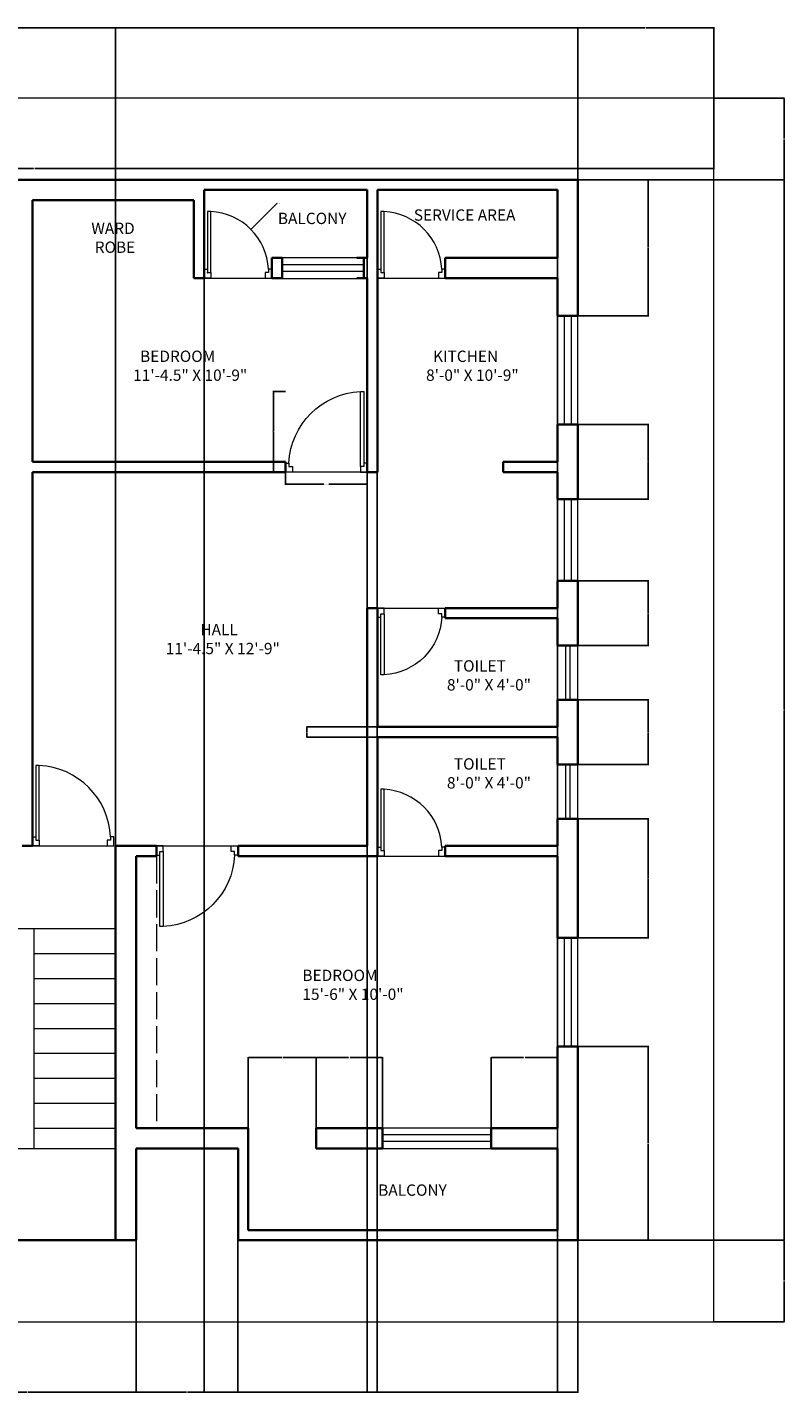
# Model space of a CAD drawing. Units: inches. Extents: x 3263 to 3926, y 954 to 1556.
# Tile 3 of 3: x 3592 to 3926, y 954 to 1556. Entities that reach past the tile are written whole.
import ezdxf

# ---------------------------------------------------------------- set-up
doc = ezdxf.new("R2010")
doc.units = ezdxf.units.IN
doc.linetypes.add('ACAD_ISO02W100', pattern=[15, 12, -3])
for name, color, linetype, lineweight in [('A-ANNO-DIMS', 2, 'Continuous', 18), ('A-ANNO-TEXT', 7, 'Continuous', 18), ('A-AREA-IDEN', 7, 'Continuous', 18), ('A-FLOR-OVHD', 8, 'ACAD_ISO02W100', 13), ('C-PROP', 8, 'Continuous', 18), ('door', 30, 'Continuous', 18), ('staircase', 31, 'Continuous', 18), ('ventilator', 210, 'Continuous', 18), ('wall', 7, 'Continuous', 35), ('window', 92, 'Continuous', 18)]:
    doc.layers.add(name, color=color, linetype=linetype, lineweight=lineweight)
doc.styles.get("Standard").update_dxf_attribs({"font": 'arial.ttf'})
doc.dimstyles.get("Standard").update_dxf_attribs({"dimtxt": 0.18, "dimasz": 0.18, "dimexe": 0.18, "dimexo": 0.0625, "dimgap": 0.09, "dimtad": 0, "dimtih": 1, "dimtoh": 1, "dimdec": 4, "dimzin": 0, "dimdsep": 46, "dimtxsty": 'Standard', "dimcen": 0.09, "dimadec": 0, "dimazin": 0, "dimtfac": 1, "dimtdec": 4, "dimtofl": 0, "dimtmove": 0, "dimatfit": 3, "dimfxl": 1, "dimtolj": 1, "dimtzin": 0, "dimarcsym": 0})

# ---------------------------------------------------------------- blocks, each defined once
blk = doc.blocks.new('d1')
at = {"layer": 'door'}
blk.add_line((4131.56, 1272.79), (4167.56, 1272.79), dxfattribs=at)
blk.add_lwpolyline([(4133.06, 1275.29), (4134.56, 1275.29), (4134.56, 1308.29), (4133.06, 1308.29)], close=True, dxfattribs=at)
for points in [[(4134.56, 1272.79), (4131.56, 1272.79), (4131.56, 1276.79), (4133.06, 1276.79), (4133.06, 1275.29), (4134.56, 1275.29), (4134.56, 1272.79)], [(4164.56, 1272.79), (4167.56, 1272.79), (4167.56, 1276.79), (4166.06, 1276.79), (4166.06, 1275.29), (4164.56, 1275.29), (4164.56, 1272.79)]]:
    blk.add_lwpolyline(points, dxfattribs=at)
blk.add_arc((4133.06, 1275.29), 33.03, 2.60256, 87.39744, dxfattribs=at)
blk = doc.blocks.new('w1')
at = {"layer": 'window'}
for p, q in [((3981.35, 1421.04), (3981.35, 1373.04)), ((3984.35, 1421.04), (3984.35, 1373.04))]:
    blk.add_line(p, q, dxfattribs=at)
blk.add_lwpolyline([(3978.35, 1373.04), (3987.35, 1373.04), (3987.35, 1421.04), (3978.35, 1421.04)], close=True, dxfattribs=at)
blk = doc.blocks.new('w2')
at = {"layer": 'window'}
for p, q in [((4050.84, 1450.41), (4050.84, 1414.41)), ((4053.84, 1450.41), (4053.84, 1414.41))]:
    blk.add_line(p, q, dxfattribs=at)
blk.add_lwpolyline([(4047.84, 1414.41), (4056.84, 1414.41), (4056.84, 1450.41), (4047.84, 1450.41)], close=True, dxfattribs=at)
blk = doc.blocks.new('d2')
at = {"layer": 'door'}
blk.add_line((4131.56, 1215.38), (4161.56, 1215.38), dxfattribs=at)
blk.add_lwpolyline([(4133.06, 1217.88), (4134.56, 1217.88), (4134.56, 1244.88), (4133.06, 1244.88)], close=True, dxfattribs=at)
for points in [[(4134.56, 1215.38), (4131.56, 1215.38), (4131.56, 1219.38), (4133.06, 1219.38), (4133.06, 1217.88), (4134.56, 1217.88), (4134.56, 1215.38)], [(4158.56, 1215.38), (4161.56, 1215.38), (4161.56, 1219.38), (4160.06, 1219.38), (4160.06, 1217.88), (4158.56, 1217.88), (4158.56, 1215.38)]]:
    blk.add_lwpolyline(points, dxfattribs=at)
blk.add_arc((4133.06, 1217.88), 27.04, 3.17983, 86.82017, dxfattribs=at)
blk = doc.blocks.new('v')
at = {"layer": 'ventilator'}
for p, q in [((4001.32, 1413.1), (4001.32, 1389.1)), ((4003.32, 1413.1), (4003.32, 1389.1))]:
    blk.add_line(p, q, dxfattribs=at)
blk.add_lwpolyline([(3997.82, 1389.1), (4006.82, 1389.1), (4006.82, 1413.1), (3997.82, 1413.1)], close=True, dxfattribs=at)
blk = doc.blocks.new('*D6')
at = {"layer": 'A-ANNO-DIMS', "color": 0, "lineweight": -2, "transparency": 16777216}
for p, q in [((3705.67, 1359.87), (3705.67, 1354.35)), ((3741.67, 1359.87), (3741.67, 1354.35)), ((3705.85, 1354.53), (3722.54, 1354.53)), ((3741.49, 1354.53), (3724.81, 1354.53))]:
    blk.add_line(p, q, dxfattribs=at)
at = {"layer": 'A-ANNO-DIMS', "color": 0, "transparency": 16777216}
for points in [[(3705.85, 1354.56), (3705.85, 1354.5), (3705.67, 1354.53)], [(3741.49, 1354.56), (3741.49, 1354.5), (3741.67, 1354.53)]]:
    blk.add_solid(points, dxfattribs=at)
at = {"layer": 'Defpoints', "color": 0, "transparency": 16777216}
for p in [(3705.67, 1359.93), (3741.67, 1359.93), (3705.67, 1354.53)]:
    blk.add_point(p, dxfattribs=at)
at = {"layer": 'A-ANNO-DIMS', "color": 0, "transparency": 16777216, "insert": (3723.67, 1354.53), "char_height": 0.18, "attachment_point": 5}
blk.add_mtext('\\A1;DOOR D1 36 TYP.', dxfattribs=at)
blk = doc.blocks.new('*D7')
at = {"layer": 'A-ANNO-DIMS', "color": 0, "lineweight": -2, "transparency": 16777216}
for p, q in [((3705.61, 1395.43), (3700.09, 1395.43)), ((3700.27, 1395.25), (3700.27, 1377.86)), ((3700.27, 1360.11), (3700.27, 1377.5)), ((3705.61, 1359.93), (3700.09, 1359.93))]:
    blk.add_line(p, q, dxfattribs=at)
at = {"layer": 'A-ANNO-DIMS', "color": 0, "transparency": 16777216}
for points in [[(3700.24, 1395.25), (3700.3, 1395.25), (3700.27, 1395.43)], [(3700.24, 1360.11), (3700.3, 1360.11), (3700.27, 1359.93)]]:
    blk.add_solid(points, dxfattribs=at)
at = {"layer": 'Defpoints', "color": 0, "transparency": 16777216}
for p in [(3700.27, 1395.43), (3705.67, 1395.43), (3705.67, 1359.93)]:
    blk.add_point(p, dxfattribs=at)
at = {"layer": 'A-ANNO-DIMS', "color": 0, "transparency": 16777216, "insert": (3700.27, 1377.68), "char_height": 0.18, "attachment_point": 5}
blk.add_mtext('\\A1;36 TYP.', dxfattribs=at)
blk = doc.blocks.new('*D16')
at = {"layer": 'A-ANNO-DIMS', "color": 0, "lineweight": -2, "transparency": 16777216}
for p, q in [((3294.67, 1524.87), (3294.67, 1493.65)), ((3894.67, 1524.87), (3894.67, 1493.65)), ((3294.85, 1493.83), (3594.39, 1493.83)), ((3894.49, 1493.83), (3594.96, 1493.83))]:
    blk.add_line(p, q, dxfattribs=at)
at = {"layer": 'A-ANNO-DIMS', "color": 0, "transparency": 16777216}
for points in [[(3294.85, 1493.86), (3294.85, 1493.8), (3294.67, 1493.83)], [(3894.49, 1493.86), (3894.49, 1493.8), (3894.67, 1493.83)]]:
    blk.add_solid(points, dxfattribs=at)
at = {"layer": 'Defpoints', "color": 0, "transparency": 16777216}
for p in [(3294.67, 1524.93), (3894.67, 1524.93), (3294.67, 1493.83)]:
    blk.add_point(p, dxfattribs=at)
at = {"layer": 'A-ANNO-DIMS', "color": 0, "transparency": 16777216, "insert": (3594.67, 1493.83), "char_height": 0.18, "attachment_point": 5}
blk.add_mtext('\\A1;600', dxfattribs=at)
blk = doc.blocks.new('*D19')
at = {"layer": 'A-ANNO-DIMS', "color": 0, "lineweight": -2, "transparency": 16777216}
for p, q in [((3318.67, 1454.49), (3318.67, 1556.21)), ((3318.85, 1556.03), (3576.39, 1556.03)), ((3834.49, 1556.03), (3576.96, 1556.03)), ((3834.67, 1488.99), (3834.67, 1556.21))]:
    blk.add_line(p, q, dxfattribs=at)
at = {"layer": 'A-ANNO-DIMS', "color": 0, "transparency": 16777216}
for points in [[(3318.85, 1556.06), (3318.85, 1556), (3318.67, 1556.03)], [(3834.49, 1556.06), (3834.49, 1556), (3834.67, 1556.03)]]:
    blk.add_solid(points, dxfattribs=at)
at = {"layer": 'Defpoints', "color": 0, "transparency": 16777216}
for p in [(3834.67, 1556.03), (3834.67, 1488.93), (3318.67, 1454.43)]:
    blk.add_point(p, dxfattribs=at)
at = {"layer": 'A-ANNO-DIMS', "color": 0, "transparency": 16777216, "insert": (3576.67, 1556.03), "char_height": 0.18, "attachment_point": 5}
blk.add_mtext('\\A1;516', dxfattribs=at)
blk = doc.blocks.new('*D20')
at = {"layer": 'A-ANNO-DIMS', "color": 0, "lineweight": -2, "transparency": 16777216}
for p, q in [((3834.67, 1488.99), (3834.67, 1556.21)), ((3834.85, 1556.03), (3864.46, 1556.03)), ((3894.49, 1556.03), (3864.89, 1556.03)), ((3894.67, 1524.99), (3894.67, 1556.21))]:
    blk.add_line(p, q, dxfattribs=at)
at = {"layer": 'A-ANNO-DIMS', "color": 0, "transparency": 16777216}
for points in [[(3834.85, 1556.06), (3834.85, 1556), (3834.67, 1556.03)], [(3894.49, 1556.06), (3894.49, 1556), (3894.67, 1556.03)]]:
    blk.add_solid(points, dxfattribs=at)
at = {"layer": 'Defpoints', "color": 0, "transparency": 16777216}
for p in [(3894.67, 1556.03), (3894.67, 1524.93), (3834.67, 1488.93)]:
    blk.add_point(p, dxfattribs=at)
at = {"layer": 'A-ANNO-DIMS', "color": 0, "transparency": 16777216, "insert": (3864.67, 1556.03), "char_height": 0.18, "attachment_point": 5}
blk.add_mtext('\\A1;60', dxfattribs=at)
blk = doc.blocks.new('*D21')
at = {"layer": 'A-ANNO-DIMS', "color": 0, "lineweight": -2, "transparency": 16777216}
for p, q in [((3834.74, 1020.93), (3925.95, 1020.93)), ((3925.77, 1020.75), (3925.77, 1003.11)), ((3925.77, 985.11), (3925.77, 1002.75)), ((3894.74, 984.93), (3925.95, 984.93))]:
    blk.add_line(p, q, dxfattribs=at)
at = {"layer": 'A-ANNO-DIMS', "color": 0, "transparency": 16777216}
for points in [[(3925.74, 1020.75), (3925.8, 1020.75), (3925.77, 1020.93)], [(3925.74, 985.11), (3925.8, 985.11), (3925.77, 984.93)]]:
    blk.add_solid(points, dxfattribs=at)
at = {"layer": 'Defpoints', "color": 0, "transparency": 16777216}
for p in [(3834.67, 1020.93), (3894.67, 984.93), (3925.77, 984.93)]:
    blk.add_point(p, dxfattribs=at)
at = {"layer": 'A-ANNO-DIMS', "color": 0, "transparency": 16777216, "insert": (3925.77, 1002.93), "char_height": 0.18, "attachment_point": 5}
blk.add_mtext('\\A1;36', dxfattribs=at)
blk = doc.blocks.new('*D22')
at = {"layer": 'A-ANNO-DIMS', "color": 0, "lineweight": -2, "transparency": 16777216}
for p, q in [((3834.74, 1488.93), (3925.95, 1488.93)), ((3925.77, 1488.75), (3925.77, 1255.11)), ((3925.77, 1021.11), (3925.77, 1254.75)), ((3834.74, 1020.93), (3925.95, 1020.93))]:
    blk.add_line(p, q, dxfattribs=at)
at = {"layer": 'A-ANNO-DIMS', "color": 0, "transparency": 16777216}
for points in [[(3925.74, 1488.75), (3925.8, 1488.75), (3925.77, 1488.93)], [(3925.74, 1021.11), (3925.8, 1021.11), (3925.77, 1020.93)]]:
    blk.add_solid(points, dxfattribs=at)
at = {"layer": 'Defpoints', "color": 0, "transparency": 16777216}
for p in [(3834.67, 1488.93), (3925.77, 1488.93), (3834.67, 1020.93)]:
    blk.add_point(p, dxfattribs=at)
at = {"layer": 'A-ANNO-DIMS', "color": 0, "transparency": 16777216, "insert": (3925.77, 1254.93), "char_height": 0.18, "attachment_point": 5}
blk.add_mtext('\\A1;468', dxfattribs=at)
blk = doc.blocks.new('*D23')
at = {"layer": 'A-ANNO-DIMS', "color": 0, "lineweight": -2, "transparency": 16777216}
for p, q in [((3894.74, 1524.93), (3925.95, 1524.93)), ((3925.77, 1524.75), (3925.77, 1507.11)), ((3925.77, 1489.11), (3925.77, 1506.75)), ((3834.74, 1488.93), (3925.95, 1488.93))]:
    blk.add_line(p, q, dxfattribs=at)
at = {"layer": 'A-ANNO-DIMS', "color": 0, "transparency": 16777216}
for points in [[(3925.74, 1524.75), (3925.8, 1524.75), (3925.77, 1524.93)], [(3925.74, 1489.11), (3925.8, 1489.11), (3925.77, 1488.93)]]:
    blk.add_solid(points, dxfattribs=at)
at = {"layer": 'Defpoints', "color": 0, "transparency": 16777216}
for p in [(3894.67, 1524.93), (3925.77, 1524.93), (3834.67, 1488.93)]:
    blk.add_point(p, dxfattribs=at)
at = {"layer": 'A-ANNO-DIMS', "color": 0, "transparency": 16777216, "insert": (3925.77, 1506.93), "char_height": 0.18, "attachment_point": 5}
blk.add_mtext('\\A1;36', dxfattribs=at)
blk = doc.blocks.new('*D26')
at = {"layer": 'A-ANNO-DIMS', "color": 0, "lineweight": -2, "transparency": 16777216}
for p, q in [((3543.67, 1020.87), (3543.67, 953.65)), ((3639.67, 1020.87), (3639.67, 953.65)), ((3543.85, 953.83), (3591.46, 953.83)), ((3639.49, 953.83), (3591.89, 953.83))]:
    blk.add_line(p, q, dxfattribs=at)
at = {"layer": 'A-ANNO-DIMS', "color": 0, "transparency": 16777216}
for points in [[(3543.85, 953.86), (3543.85, 953.8), (3543.67, 953.83)], [(3639.49, 953.86), (3639.49, 953.8), (3639.67, 953.83)]]:
    blk.add_solid(points, dxfattribs=at)
at = {"layer": 'Defpoints', "color": 0, "transparency": 16777216}
for p in [(3543.67, 1020.93), (3639.67, 1020.93), (3639.67, 953.83)]:
    blk.add_point(p, dxfattribs=at)
at = {"layer": 'A-ANNO-DIMS', "color": 0, "transparency": 16777216, "insert": (3591.67, 953.83), "char_height": 0.18, "attachment_point": 5}
blk.add_mtext('\\A1;96', dxfattribs=at)
blk = doc.blocks.new('*D27')
at = {"layer": 'A-ANNO-DIMS', "color": 0, "lineweight": -2, "transparency": 16777216}
for p, q in [((3639.67, 1020.87), (3639.67, 953.65)), ((3684.67, 1020.87), (3684.67, 953.65)), ((3639.85, 953.83), (3661.95, 953.83)), ((3684.49, 953.83), (3662.4, 953.83))]:
    blk.add_line(p, q, dxfattribs=at)
at = {"layer": 'A-ANNO-DIMS', "color": 0, "transparency": 16777216}
for points in [[(3639.85, 953.86), (3639.85, 953.8), (3639.67, 953.83)], [(3684.49, 953.86), (3684.49, 953.8), (3684.67, 953.83)]]:
    blk.add_solid(points, dxfattribs=at)
at = {"layer": 'Defpoints', "color": 0, "transparency": 16777216}
for p in [(3639.67, 1020.93), (3684.67, 1020.93), (3684.67, 953.83)]:
    blk.add_point(p, dxfattribs=at)
at = {"layer": 'A-ANNO-DIMS', "color": 0, "transparency": 16777216, "insert": (3662.17, 953.83), "char_height": 0.18, "attachment_point": 5}
blk.add_mtext('\\A1;45', dxfattribs=at)
blk = doc.blocks.new('*D28')
at = {"layer": 'A-ANNO-DIMS', "color": 0, "lineweight": -2, "transparency": 16777216}
for p, q in [((3684.67, 1020.87), (3684.67, 953.65)), ((3834.67, 1020.87), (3834.67, 953.65)), ((3684.85, 953.83), (3759.39, 953.83)), ((3834.49, 953.83), (3759.95, 953.83))]:
    blk.add_line(p, q, dxfattribs=at)
at = {"layer": 'A-ANNO-DIMS', "color": 0, "transparency": 16777216}
for points in [[(3684.85, 953.86), (3684.85, 953.8), (3684.67, 953.83)], [(3834.49, 953.86), (3834.49, 953.8), (3834.67, 953.83)]]:
    blk.add_solid(points, dxfattribs=at)
at = {"layer": 'Defpoints', "color": 0, "transparency": 16777216}
for p in [(3684.67, 1020.93), (3834.67, 1020.93), (3834.67, 953.83)]:
    blk.add_point(p, dxfattribs=at)
at = {"layer": 'A-ANNO-DIMS', "color": 0, "transparency": 16777216, "insert": (3759.67, 953.83), "char_height": 0.18, "attachment_point": 5}
blk.add_mtext('\\A1;150', dxfattribs=at)
blk = doc.blocks.new('*D29')
at = {"layer": 'A-ANNO-DIMS', "color": 0, "lineweight": -2, "transparency": 16777216}
for p, q in [((3552.67, 1020.99), (3552.67, 1556.21)), ((3552.85, 1556.03), (3591.46, 1556.03)), ((3630.49, 1556.03), (3591.89, 1556.03)), ((3630.67, 1020.99), (3630.67, 1556.21))]:
    blk.add_line(p, q, dxfattribs=at)
at = {"layer": 'A-ANNO-DIMS', "color": 0, "transparency": 16777216}
for points in [[(3552.85, 1556.06), (3552.85, 1556), (3552.67, 1556.03)], [(3630.49, 1556.06), (3630.49, 1556), (3630.67, 1556.03)]]:
    blk.add_solid(points, dxfattribs=at)
at = {"layer": 'Defpoints', "color": 0, "transparency": 16777216}
for p in [(3630.67, 1556.03), (3552.67, 1020.93), (3630.67, 1020.93)]:
    blk.add_point(p, dxfattribs=at)
at = {"layer": 'A-ANNO-DIMS', "color": 0, "transparency": 16777216, "insert": (3591.67, 1556.03), "char_height": 0.18, "attachment_point": 5}
blk.add_mtext('\\A1;78', dxfattribs=at)
blk = doc.blocks.new('*D39')
at = {"layer": 'A-ANNO-DIMS', "color": 0, "lineweight": -2, "transparency": 16777216}
for p, q in [((3669.67, 1484.37), (3669.67, 953.65)), ((3741.67, 1484.37), (3741.67, 953.65)), ((3669.85, 953.83), (3705.46, 953.83)), ((3741.49, 953.83), (3705.89, 953.83))]:
    blk.add_line(p, q, dxfattribs=at)
at = {"layer": 'A-ANNO-DIMS', "color": 0, "transparency": 16777216}
for points in [[(3669.85, 953.86), (3669.85, 953.8), (3669.67, 953.83)], [(3741.49, 953.86), (3741.49, 953.8), (3741.67, 953.83)]]:
    blk.add_solid(points, dxfattribs=at)
at = {"layer": 'Defpoints', "color": 0, "transparency": 16777216}
for p in [(3669.67, 1484.43), (3741.67, 1484.43), (3741.67, 953.83)]:
    blk.add_point(p, dxfattribs=at)
at = {"layer": 'A-ANNO-DIMS', "color": 0, "transparency": 16777216, "insert": (3705.67, 953.83), "char_height": 0.18, "attachment_point": 5}
blk.add_mtext('\\A1;72', dxfattribs=at)
blk = doc.blocks.new('*D40')
at = {"layer": 'A-ANNO-DIMS', "color": 0, "lineweight": -2, "transparency": 16777216}
for p, q in [((3746.17, 1484.37), (3746.17, 953.65)), ((3825.67, 1484.37), (3825.67, 953.65)), ((3746.35, 953.83), (3785.6, 953.83)), ((3825.49, 953.83), (3786.25, 953.83))]:
    blk.add_line(p, q, dxfattribs=at)
at = {"layer": 'A-ANNO-DIMS', "color": 0, "transparency": 16777216}
for points in [[(3746.35, 953.86), (3746.35, 953.8), (3746.17, 953.83)], [(3825.49, 953.86), (3825.49, 953.8), (3825.67, 953.83)]]:
    blk.add_solid(points, dxfattribs=at)
at = {"layer": 'Defpoints', "color": 0, "transparency": 16777216}
for p in [(3746.17, 1484.43), (3825.67, 1484.43), (3825.67, 953.83)]:
    blk.add_point(p, dxfattribs=at)
at = {"layer": 'A-ANNO-DIMS', "color": 0, "transparency": 16777216, "insert": (3785.92, 953.83), "char_height": 0.18, "attachment_point": 5}
blk.add_mtext('\\A1;79.5', dxfattribs=at)
blk = doc.blocks.new('*D41')
at = {"layer": 'A-ANNO-DIMS', "color": 0, "lineweight": -2, "transparency": 16777216}
for p, q in [((3834.74, 1488.93), (3865.95, 1488.93)), ((3865.77, 1488.75), (3865.77, 1459.11)), ((3865.77, 1429.11), (3865.77, 1458.75)), ((3834.74, 1428.93), (3865.95, 1428.93))]:
    blk.add_line(p, q, dxfattribs=at)
at = {"layer": 'A-ANNO-DIMS', "color": 0, "transparency": 16777216}
for points in [[(3865.74, 1488.75), (3865.8, 1488.75), (3865.77, 1488.93)], [(3865.74, 1429.11), (3865.8, 1429.11), (3865.77, 1428.93)]]:
    blk.add_solid(points, dxfattribs=at)
at = {"layer": 'Defpoints', "color": 0, "transparency": 16777216}
for p in [(3834.67, 1488.93), (3834.67, 1428.93), (3865.77, 1428.93)]:
    blk.add_point(p, dxfattribs=at)
at = {"layer": 'A-ANNO-DIMS', "color": 0, "transparency": 16777216, "insert": (3865.77, 1458.93), "char_height": 0.18, "attachment_point": 5}
blk.add_mtext('\\A1;60', dxfattribs=at)
blk = doc.blocks.new('*D42')
at = {"layer": 'A-ANNO-DIMS', "color": 0, "lineweight": -2, "transparency": 16777216}
for p, q in [((3834.74, 1380.93), (3865.95, 1380.93)), ((3865.77, 1380.75), (3865.77, 1364.61)), ((3865.77, 1348.11), (3865.77, 1364.25)), ((3834.74, 1347.93), (3865.95, 1347.93))]:
    blk.add_line(p, q, dxfattribs=at)
at = {"layer": 'A-ANNO-DIMS', "color": 0, "transparency": 16777216}
for points in [[(3865.74, 1380.75), (3865.8, 1380.75), (3865.77, 1380.93)], [(3865.74, 1348.11), (3865.8, 1348.11), (3865.77, 1347.93)]]:
    blk.add_solid(points, dxfattribs=at)
at = {"layer": 'Defpoints', "color": 0, "transparency": 16777216}
for p in [(3834.67, 1380.93), (3834.67, 1347.93), (3865.77, 1347.93)]:
    blk.add_point(p, dxfattribs=at)
at = {"layer": 'A-ANNO-DIMS', "color": 0, "transparency": 16777216, "insert": (3865.77, 1364.43), "char_height": 0.18, "attachment_point": 5}
blk.add_mtext('\\A1;33', dxfattribs=at)
blk = doc.blocks.new('*D43')
at = {"layer": 'A-ANNO-DIMS', "color": 0, "lineweight": -2, "transparency": 16777216}
for p, q in [((3834.74, 1311.93), (3865.95, 1311.93)), ((3865.77, 1311.75), (3865.77, 1297.86)), ((3865.77, 1283.61), (3865.77, 1297.5)), ((3834.74, 1283.43), (3865.95, 1283.43))]:
    blk.add_line(p, q, dxfattribs=at)
at = {"layer": 'A-ANNO-DIMS', "color": 0, "transparency": 16777216}
for points in [[(3865.74, 1311.75), (3865.8, 1311.75), (3865.77, 1311.93)], [(3865.74, 1283.61), (3865.8, 1283.61), (3865.77, 1283.43)]]:
    blk.add_solid(points, dxfattribs=at)
at = {"layer": 'Defpoints', "color": 0, "transparency": 16777216}
for p in [(3834.67, 1311.93), (3834.67, 1283.43), (3865.77, 1283.43)]:
    blk.add_point(p, dxfattribs=at)
at = {"layer": 'A-ANNO-DIMS', "color": 0, "transparency": 16777216, "insert": (3865.77, 1297.68), "char_height": 0.18, "attachment_point": 5}
blk.add_mtext('\\A1;28.5', dxfattribs=at)
blk = doc.blocks.new('*D44')
at = {"layer": 'A-ANNO-DIMS', "color": 0, "lineweight": -2, "transparency": 16777216}
for p, q in [((3834.74, 1259.43), (3865.95, 1259.43)), ((3865.77, 1259.25), (3865.77, 1245.36)), ((3865.77, 1231.11), (3865.77, 1245)), ((3834.74, 1230.93), (3865.95, 1230.93))]:
    blk.add_line(p, q, dxfattribs=at)
at = {"layer": 'A-ANNO-DIMS', "color": 0, "transparency": 16777216}
for points in [[(3865.74, 1259.25), (3865.8, 1259.25), (3865.77, 1259.43)], [(3865.74, 1231.11), (3865.8, 1231.11), (3865.77, 1230.93)]]:
    blk.add_solid(points, dxfattribs=at)
at = {"layer": 'Defpoints', "color": 0, "transparency": 16777216}
for p in [(3834.67, 1259.43), (3834.67, 1230.93), (3865.77, 1230.93)]:
    blk.add_point(p, dxfattribs=at)
at = {"layer": 'A-ANNO-DIMS', "color": 0, "transparency": 16777216, "insert": (3865.77, 1245.18), "char_height": 0.18, "attachment_point": 5}
blk.add_mtext('\\A1;28.5', dxfattribs=at)
blk = doc.blocks.new('*D45')
at = {"layer": 'A-ANNO-DIMS', "color": 0, "lineweight": -2, "transparency": 16777216}
for p, q in [((3834.74, 1206.93), (3865.95, 1206.93)), ((3865.77, 1206.75), (3865.77, 1180.86)), ((3865.77, 1154.61), (3865.77, 1180.5)), ((3834.74, 1154.43), (3865.95, 1154.43))]:
    blk.add_line(p, q, dxfattribs=at)
at = {"layer": 'A-ANNO-DIMS', "color": 0, "transparency": 16777216}
for points in [[(3865.74, 1206.75), (3865.8, 1206.75), (3865.77, 1206.93)], [(3865.74, 1154.61), (3865.8, 1154.61), (3865.77, 1154.43)]]:
    blk.add_solid(points, dxfattribs=at)
at = {"layer": 'Defpoints', "color": 0, "transparency": 16777216}
for p in [(3834.67, 1206.93), (3834.67, 1154.43), (3865.77, 1154.43)]:
    blk.add_point(p, dxfattribs=at)
at = {"layer": 'A-ANNO-DIMS', "color": 0, "transparency": 16777216, "insert": (3865.77, 1180.68), "char_height": 0.18, "attachment_point": 5}
blk.add_mtext('\\A1;52.5', dxfattribs=at)
blk = doc.blocks.new('*D46')
at = {"layer": 'A-ANNO-DIMS', "color": 0, "lineweight": -2, "transparency": 16777216}
for p, q in [((3834.74, 1106.43), (3865.95, 1106.43)), ((3865.77, 1106.25), (3865.77, 1063.86)), ((3865.77, 1021.11), (3865.77, 1063.5)), ((3834.74, 1020.93), (3865.95, 1020.93))]:
    blk.add_line(p, q, dxfattribs=at)
at = {"layer": 'A-ANNO-DIMS', "color": 0, "transparency": 16777216}
for points in [[(3865.74, 1106.25), (3865.8, 1106.25), (3865.77, 1106.43)], [(3865.74, 1021.11), (3865.8, 1021.11), (3865.77, 1020.93)]]:
    blk.add_solid(points, dxfattribs=at)
at = {"layer": 'Defpoints', "color": 0, "transparency": 16777216}
for p in [(3834.67, 1106.43), (3834.67, 1020.93), (3865.77, 1020.93)]:
    blk.add_point(p, dxfattribs=at)
at = {"layer": 'A-ANNO-DIMS', "color": 0, "transparency": 16777216, "insert": (3865.77, 1063.68), "char_height": 0.18, "attachment_point": 5}
blk.add_mtext('\\A1;85.5', dxfattribs=at)
blk = doc.blocks.new('*D54')
at = {"layer": 'A-ANNO-DIMS', "color": 0, "lineweight": -2, "transparency": 16777216}
for p, q in [((3689.17, 1070.49), (3689.17, 1101.71)), ((3689.35, 1101.53), (3703.96, 1101.53)), ((3718.99, 1101.53), (3704.39, 1101.53)), ((3719.17, 1070.49), (3719.17, 1101.71))]:
    blk.add_line(p, q, dxfattribs=at)
at = {"layer": 'A-ANNO-DIMS', "color": 0, "transparency": 16777216}
for points in [[(3689.35, 1101.56), (3689.35, 1101.5), (3689.17, 1101.53)], [(3718.99, 1101.56), (3718.99, 1101.5), (3719.17, 1101.53)]]:
    blk.add_solid(points, dxfattribs=at)
at = {"layer": 'Defpoints', "color": 0, "transparency": 16777216}
for p in [(3719.17, 1101.53), (3689.17, 1070.43), (3719.17, 1070.43)]:
    blk.add_point(p, dxfattribs=at)
at = {"layer": 'A-ANNO-DIMS', "color": 0, "transparency": 16777216, "insert": (3704.17, 1101.53), "char_height": 0.18, "attachment_point": 5}
blk.add_mtext('\\A1;30', dxfattribs=at)
blk = doc.blocks.new('*D55')
at = {"layer": 'A-ANNO-DIMS', "color": 0, "lineweight": -2, "transparency": 16777216}
for p, q in [((3719.17, 1070.49), (3719.17, 1101.71)), ((3719.35, 1101.53), (3733.4, 1101.53)), ((3748.24, 1101.53), (3734.2, 1101.53)), ((3748.42, 1070.49), (3748.42, 1101.71))]:
    blk.add_line(p, q, dxfattribs=at)
at = {"layer": 'A-ANNO-DIMS', "color": 0, "transparency": 16777216}
for points in [[(3719.35, 1101.56), (3719.35, 1101.5), (3719.17, 1101.53)], [(3748.24, 1101.56), (3748.24, 1101.5), (3748.42, 1101.53)]]:
    blk.add_solid(points, dxfattribs=at)
at = {"layer": 'Defpoints', "color": 0, "transparency": 16777216}
for p in [(3748.42, 1101.53), (3719.17, 1070.43), (3748.42, 1070.43)]:
    blk.add_point(p, dxfattribs=at)
at = {"layer": 'A-ANNO-DIMS', "color": 0, "transparency": 16777216, "insert": (3733.8, 1101.53), "char_height": 0.18, "attachment_point": 5}
blk.add_mtext('\\A1;29.25', dxfattribs=at)
blk = doc.blocks.new('*D56')
at = {"layer": 'A-ANNO-DIMS', "color": 0, "lineweight": -2, "transparency": 16777216}
for p, q in [((3796.42, 1070.49), (3796.42, 1101.71)), ((3796.6, 1101.53), (3810.65, 1101.53)), ((3825.49, 1101.53), (3811.45, 1101.53)), ((3825.67, 1070.49), (3825.67, 1101.71))]:
    blk.add_line(p, q, dxfattribs=at)
at = {"layer": 'A-ANNO-DIMS', "color": 0, "transparency": 16777216}
for points in [[(3796.6, 1101.56), (3796.6, 1101.5), (3796.42, 1101.53)], [(3825.49, 1101.56), (3825.49, 1101.5), (3825.67, 1101.53)]]:
    blk.add_solid(points, dxfattribs=at)
at = {"layer": 'Defpoints', "color": 0, "transparency": 16777216}
for p in [(3825.67, 1101.53), (3796.42, 1070.43), (3825.67, 1070.43)]:
    blk.add_point(p, dxfattribs=at)
at = {"layer": 'A-ANNO-DIMS', "color": 0, "transparency": 16777216, "insert": (3811.05, 1101.53), "char_height": 0.18, "attachment_point": 5}
blk.add_mtext('\\A1;29.25', dxfattribs=at)
blk = doc.blocks.new('*D57')
at = {"layer": 'A-ANNO-DIMS', "color": 0, "lineweight": -2, "transparency": 16777216}
for p, q in [((3746.11, 1247.43), (3714.89, 1247.43)), ((3746.11, 1242.93), (3714.89, 1242.93)), ((3715.07, 1247.25), (3715.07, 1245.36)), ((3715.07, 1243.11), (3715.07, 1245))]:
    blk.add_line(p, q, dxfattribs=at)
at = {"layer": 'A-ANNO-DIMS', "color": 0, "transparency": 16777216}
for points in [[(3715.04, 1247.25), (3715.1, 1247.25), (3715.07, 1247.43)], [(3715.04, 1243.11), (3715.1, 1243.11), (3715.07, 1242.93)]]:
    blk.add_solid(points, dxfattribs=at)
at = {"layer": 'Defpoints', "color": 0, "transparency": 16777216}
for p in [(3715.07, 1247.43), (3746.17, 1247.43), (3746.17, 1242.93)]:
    blk.add_point(p, dxfattribs=at)
at = {"layer": 'A-ANNO-DIMS', "color": 0, "transparency": 16777216, "insert": (3715.07, 1245.18), "char_height": 0.18, "attachment_point": 5}
blk.add_mtext('\\A1;4.5', dxfattribs=at)
blk = doc.blocks.new('*D59')
at = {"layer": 'A-ANNO-DIMS', "color": 0, "lineweight": -2, "transparency": 16777216}
for p, q in [((3701.77, 1478.52), (3690.42, 1467.18)), ((3701.95, 1478.52), (3701.77, 1478.52)), ((3671.08, 1447.93), (3671.26, 1447.93)), ((3671.17, 1447.84), (3671.17, 1448.02))]:
    blk.add_line(p, q, dxfattribs=at)
at = {"layer": 'A-ANNO-DIMS', "color": 0, "transparency": 16777216}
blk.add_solid([(3690.4, 1467.2), (3690.44, 1467.16), (3690.3, 1467.05)], dxfattribs=at)
at = {"layer": 'Defpoints', "color": 0, "transparency": 16777216}
for p in [(3690.3, 1467.05), (3671.17, 1447.93)]:
    blk.add_point(p, dxfattribs=at)
at = {"layer": 'A-ANNO-DIMS', "color": 0, "transparency": 16777216, "insert": (3702.62, 1478.52), "char_height": 0.18, "attachment_point": 5}
blk.add_mtext('\\A1;9X R27.04', dxfattribs=at)

msp = doc.modelspace()

# ---------------------------------------------------------------- linework, layer by layer
at = {"layer": 'A-FLOR-OVHD'}
msp.add_line((3648.6743, 1190.4303), (3648.6743, 1070.4303), dxfattribs=at)
at = {"layer": 'C-PROP'}
for p, q in [((3894.6743, 1524.9303), (3294.6743, 1524.9303)), ((3894.6743, 984.9303), (3894.6743, 1524.9303)), ((3294.6743, 984.9303), (3894.6743, 984.9303))]:
    msp.add_line(p, q, dxfattribs=at)
at = {"layer": 'staircase'}
for p, q in [((3552.6743, 1158.4303), (3630.6743, 1158.4303)), ((3594.6743, 1061.4303), (3594.6743, 1158.4303)), ((3594.6743, 1147.4303), (3630.6743, 1147.4303)), ((3594.6743, 1136.4303), (3630.6743, 1136.4303)), ((3594.6743, 1125.4303), (3630.6743, 1125.4303)), ((3594.6743, 1114.4303), (3630.6743, 1114.4303)), ((3594.6743, 1103.4303), (3630.6743, 1103.4303)), ((3594.6743, 1092.4303), (3630.6743, 1092.4303)), ((3594.6743, 1081.4303), (3630.6743, 1081.4303)), ((3594.6743, 1070.4303), (3630.6743, 1070.4303)), ((3552.6743, 1061.4303), (3630.6743, 1061.4303))]:
    msp.add_line(p, q, dxfattribs=at)
at = {"layer": 'wall'}
for p, q in [((3834.6743, 1488.9303), (3524.1743, 1488.9303)), ((3834.6743, 1428.9303), (3834.6743, 1488.9303)), ((3669.6743, 1484.4303), (3669.6743, 1445.4303)), ((3741.6743, 1484.4303), (3669.6743, 1484.4303)), ((3741.6743, 1484.4303), (3741.6743, 1454.4303)), ((3825.6743, 1484.4303), (3746.1743, 1484.4303)), ((3746.1743, 1484.4303), (3746.1743, 1445.4303)), ((3825.6743, 1454.4303), (3825.6743, 1484.4303)), ((3593.9243, 1479.9303), (3593.9243, 1364.4303)), ((3665.1743, 1479.9303), (3593.9243, 1479.9303)), ((3665.1743, 1479.9303), (3665.1743, 1445.4303)), ((3699.6743, 1454.4303), (3699.6743, 1445.4303)), ((3704.1743, 1454.4303), (3699.6743, 1454.4303)), ((3704.1743, 1454.4303), (3704.1743, 1445.4303)), ((3741.6743, 1454.4303), (3737.1743, 1454.4303)), ((3740.1743, 1454.4303), (3740.1743, 1445.4303)), ((3825.6743, 1454.4303), (3776.1743, 1454.4303)), ((3776.1743, 1454.4303), (3776.1743, 1445.4303)), ((3665.1743, 1445.4303), (3669.6743, 1445.4303)), ((3704.1743, 1445.4303), (3699.6743, 1445.4303)), ((3741.6743, 1445.4303), (3737.1743, 1445.4303)), ((3741.6743, 1445.4303), (3741.6743, 1359.9303)), ((3746.1743, 1445.4303), (3746.1743, 1359.9303)), ((3825.6743, 1445.4303), (3776.1743, 1445.4303)), ((3825.6743, 1428.9303), (3825.6743, 1445.4303)), ((3825.6743, 1428.9303), (3834.6743, 1428.9303)), ((3825.6743, 1364.4303), (3825.6743, 1380.9303)), ((3825.6743, 1380.9303), (3834.6743, 1380.9303)), ((3834.6743, 1347.9303), (3834.6743, 1380.9303)), ((3705.6743, 1364.4303), (3593.9243, 1364.4303)), ((3705.6743, 1364.4303), (3705.6743, 1359.9303)), ((3825.6743, 1364.4303), (3801.6743, 1364.4303)), ((3801.6743, 1364.4303), (3801.6743, 1359.9303)), ((3705.6743, 1359.9303), (3593.9243, 1359.9303)), ((3593.9243, 1359.9303), (3593.9243, 1194.9303)), ((3746.1743, 1359.9303), (3741.6743, 1359.9303)), ((3825.6743, 1359.9303), (3801.6743, 1359.9303)), ((3825.6743, 1347.9303), (3825.6743, 1359.9303)), ((3825.6743, 1347.9303), (3834.6743, 1347.9303)), ((3825.6743, 1299.9303), (3825.6743, 1311.9303)), ((3825.6743, 1311.9303), (3834.6743, 1311.9303)), ((3834.6743, 1283.4303), (3834.6743, 1311.9303)), ((3741.6743, 1299.9303), (3741.6743, 1194.9303)), ((3746.1743, 1299.9303), (3741.6743, 1299.9303)), ((3746.1743, 1299.9303), (3746.1743, 1247.4303)), ((3776.1743, 1299.9303), (3825.6743, 1299.9303)), ((3776.1743, 1299.9303), (3776.1743, 1295.4303)), ((3776.1743, 1295.4303), (3825.6743, 1295.4303)), ((3825.6743, 1283.4303), (3825.6743, 1295.4303)), ((3825.6743, 1283.4303), (3834.6743, 1283.4303)), ((3825.6743, 1247.4303), (3825.6743, 1259.4303)), ((3825.6743, 1259.4303), (3834.6743, 1259.4303)), ((3834.6743, 1230.9303), (3834.6743, 1259.4303)), ((3746.1743, 1247.4303), (3825.6743, 1247.4303)), ((3746.1743, 1242.9303), (3825.6743, 1242.9303)), ((3746.1743, 1242.9303), (3746.1743, 1190.4303)), ((3825.6743, 1230.9303), (3825.6743, 1242.9303)), ((3825.6743, 1230.9303), (3834.6743, 1230.9303)), ((3825.6743, 1194.9303), (3825.6743, 1206.9303)), ((3825.6743, 1206.9303), (3834.6743, 1206.9303)), ((3834.6743, 1154.4303), (3834.6743, 1206.9303)), ((3589.4243, 1194.9303), (3593.9243, 1194.9303)), ((3630.6743, 1194.9303), (3648.6743, 1194.9303)), ((3630.6743, 1020.9303), (3630.6743, 1194.9303)), ((3648.6743, 1190.4303), (3648.6743, 1194.9303)), ((3684.6743, 1194.9303), (3741.6743, 1194.9303)), ((3684.6743, 1190.4303), (3684.6743, 1194.9303)), ((3776.1743, 1194.9303), (3776.1743, 1190.4303)), ((3776.1743, 1194.9303), (3825.6743, 1194.9303)), ((3639.6743, 1190.4303), (3648.6743, 1190.4303)), ((3639.6743, 1070.4303), (3639.6743, 1190.4303)), ((3746.1743, 1190.4303), (3684.6743, 1190.4303)), ((3776.1743, 1190.4303), (3825.6743, 1190.4303)), ((3825.6743, 1154.4303), (3825.6743, 1190.4303)), ((3825.6743, 1154.4303), (3834.6743, 1154.4303)), ((3825.6743, 1070.4303), (3825.6743, 1106.4303)), ((3825.6743, 1106.4303), (3834.6743, 1106.4303)), ((3834.6743, 1020.9303), (3834.6743, 1106.4303)), ((3639.6743, 1070.4303), (3689.1743, 1070.4303)), ((3689.1743, 1025.4303), (3689.1743, 1070.4303)), ((3719.1743, 1061.4303), (3719.1743, 1070.4303)), ((3719.1743, 1070.4303), (3748.4243, 1070.4303)), ((3748.4243, 1061.4303), (3748.4243, 1070.4303)), ((3796.4243, 1061.4303), (3796.4243, 1070.4303)), ((3796.4243, 1070.4303), (3825.6743, 1070.4303)), ((3639.6743, 1020.9303), (3639.6743, 1061.4303)), ((3639.6743, 1061.4303), (3684.6743, 1061.4303)), ((3684.6743, 1020.9303), (3684.6743, 1061.4303)), ((3719.1743, 1061.4303), (3748.4243, 1061.4303)), ((3796.4243, 1061.4303), (3825.6743, 1061.4303)), ((3825.6743, 1025.4303), (3825.6743, 1061.4303)), ((3689.1743, 1025.4303), (3825.6743, 1025.4303)), ((3543.6743, 1020.9303), (3639.6743, 1020.9303)), ((3684.6743, 1020.9303), (3834.6743, 1020.9303))]:
    msp.add_line(p, q, dxfattribs=at)

# ---------------------------------------------------------------- block references
at = {"layer": 'door'}
for name, p in [('d2', (-461.8842, 230.0526)), ('d2', (-385.3842, 230.0526)), ('d1', (-537.6342, -77.8568)), ('d2', (-385.3842, -24.9474))]:
    msp.add_blockref(name, p, dxfattribs=at)
at = {"layer": 'door', "xscale": -1}
msp.add_blockref('d1', (7873.2328, 87.1432), dxfattribs=at)
at = {"layer": 'door', "xscale": -1, "rotation": 180}
for name, p in [('d2', (-385.3842, 2515.308)), ('d1', (-482.8842, 2467.7175))]:
    msp.add_blockref(name, p, dxfattribs=at)
at = {"layer": 'ventilator'}
for p in [(-172.1433, -129.6707), (-172.1433, -182.1707)]:
    msp.add_blockref('v', p, dxfattribs=at)
at = {"layer": 'window', "rotation": 270}
for name, p in [('w2', (2289.7656, 5502.269)), ('w1', (2375.3872, 5048.7852))]:
    msp.add_blockref(name, p, dxfattribs=at)
at = {"layer": 'window'}
for name, p in [('w1', (-152.6806, 7.8933)), ('w2', (-222.1644, -102.4784)), ('w1', (-152.6806, -266.6067))]:
    msp.add_blockref(name, p, dxfattribs=at)

# ---------------------------------------------------------------- texts
at = {"layer": 'A-ANNO-TEXT', "insert": (3619.915, 1470.0044), "char_height": 5, "attachment_point": 1}
msp.add_mtext_dynamic_manual_height_columns('WARD   ROBE', width=21.465717, gutter_width=12.5, heights=[0], dxfattribs=at)
at = {"layer": 'A-AREA-IDEN', "char_height": 5, "attachment_point": 1}
for s, width, insert in [('BALCONY', 62.092631, (3702.2717, 1474.3808)), ('SERVICE AREA', 62.092631, (3762.2705, 1475.8649)), ('  BEDROOM\\P11\'-4.5" X 10\'-9"', 60.302269, (3638.3995, 1413.5302)), ('  KITCHEN\\P8\'-0" X 10\'-9"', 42.17852, (3767.6863, 1413.5302)), ('          HALL\\P11\'-4.5" X 12\'-9"', 64.375157, (3652.7882, 1292.9009)), ('  TOILET\\P8\'-0" X 4\'-0"', 42.17852, (3776.8923, 1276.8837)), ('  TOILET\\P8\'-0" X 4\'-0"', 42.17852, (3776.8923, 1233.6239)), ('BEDROOM\\P15\'-6" X 10\'-0"', 66.66276, (3713.09, 1140.3257)), ('BALCONY', 62.092631, (3746.5475, 1045.5573))]:
    msp.add_mtext_dynamic_manual_height_columns(s, width=width, gutter_width=12.5, heights=[0], dxfattribs=dict(at, insert=insert))

# ---------------------------------------------------------------- dimensions: what is measured, and where the dimension line sits
at = {"layer": 'A-ANNO-DIMS'}
for base, p1, p2, override, picture, middle in [((3834.6743, 1556.0303), (3318.6743, 1454.4303), (3834.6743, 1488.9303), {"dimdec": 0, "dimlfac": 1, "dimrnd": 0, "dimzin": 0, "dimdsep": 46, "dimlunit": 2}, '*D19', (3576.6743, 1556.0303)), ((3630.6743, 1556.0303), (3552.6743, 1020.9303), (3630.6743, 1020.9303), {"dimdec": 0, "dimlfac": 1, "dimrnd": 0, "dimzin": 0, "dimdsep": 46, "dimlunit": 2}, '*D29', (3591.6743, 1556.0303)), ((3894.6743, 1556.0303), (3834.6743, 1488.9303), (3894.6743, 1524.9303), {"dimdec": 0, "dimlfac": 1, "dimrnd": 0, "dimzin": 0, "dimdsep": 46, "dimlunit": 2}, '*D20', (3864.6743, 1556.0303)), ((3741.6743, 953.8303), (3669.6743, 1484.4303), (3741.6743, 1484.4303), {"dimdec": 0, "dimlfac": 1, "dimrnd": 0, "dimzin": 0, "dimdsep": 46, "dimlunit": 2}, '*D39', (3705.6743, 953.8303)), ((3825.6743, 953.8303), (3746.1743, 1484.4303), (3825.6743, 1484.4303), {"dimdec": 1, "dimlfac": 1, "dimrnd": 0, "dimzin": 0, "dimdsep": 46, "dimlunit": 2}, '*D40', (3785.9243, 953.8303)), ((3719.1743, 1101.5303), (3689.1743, 1070.4303), (3719.1743, 1070.4303), {"dimdec": 0, "dimlfac": 1, "dimrnd": 0, "dimzin": 0, "dimdsep": 46, "dimlunit": 2}, '*D54', (3704.1743, 1101.5303)), ((3748.4243, 1101.5303), (3719.1743, 1070.4303), (3748.4243, 1070.4303), {"dimdec": 2, "dimlfac": 1, "dimrnd": 0, "dimzin": 0, "dimdsep": 46, "dimlunit": 2}, '*D55', (3733.7993, 1101.5303)), ((3639.6743, 953.8303), (3543.6743, 1020.9303), (3639.6743, 1020.9303), {"dimdec": 0, "dimlfac": 1, "dimrnd": 0, "dimzin": 0, "dimdsep": 46, "dimlunit": 2}, '*D26', (3591.6743, 953.8303)), ((3684.6743, 953.8303), (3639.6743, 1020.9303), (3684.6743, 1020.9303), {"dimdec": 0, "dimlfac": 1, "dimrnd": 0, "dimzin": 0, "dimdsep": 46, "dimlunit": 2}, '*D27', (3662.1743, 953.8303)), ((3834.6743, 953.8303), (3684.6743, 1020.9303), (3834.6743, 1020.9303), {"dimdec": 0, "dimlfac": 1, "dimrnd": 0, "dimzin": 0, "dimdsep": 46, "dimlunit": 2}, '*D28', (3759.6743, 953.8303))]:
    dim = msp.add_linear_dim(base=base, p1=p1, p2=p2, dimstyle='Standard', override=override, dxfattribs=at)
    dim.commit()
    dim.dimension.update_dxf_attribs({"geometry": picture, "text_midpoint": middle})
for base, p1, p2, angle, override, picture, middle in [((3294.6743, 1493.8303), (3894.6743, 1524.9303), (3294.6743, 1524.9303), 180, {"dimdec": 0, "dimlfac": 1, "dimrnd": 0, "dimzin": 0, "dimdsep": 46, "dimlunit": 2}, '*D16', (3594.6743, 1493.8303)), ((3925.7743, 1524.9303), (3834.6743, 1488.9303), (3894.6743, 1524.9303), 90, {"dimdec": 0, "dimlfac": 1, "dimrnd": 0, "dimzin": 0, "dimdsep": 46, "dimlunit": 2}, '*D23', (3925.7743, 1506.9303)), ((3925.7743, 1488.9303), (3834.6743, 1020.9303), (3834.6743, 1488.9303), 90, {"dimdec": 0, "dimlfac": 1, "dimrnd": 0, "dimzin": 0, "dimdsep": 46, "dimlunit": 2}, '*D22', (3925.7743, 1254.9303)), ((3865.7743, 1428.9303), (3834.6743, 1488.9303), (3834.6743, 1428.9303), 270, {"dimdec": 0, "dimlfac": 1, "dimrnd": 0, "dimzin": 0, "dimdsep": 46, "dimlunit": 2}, '*D41', (3865.7743, 1458.9303)), ((3865.7743, 1347.9303), (3834.6743, 1380.9303), (3834.6743, 1347.9303), 270, {"dimdec": 0, "dimlfac": 1, "dimrnd": 0, "dimzin": 0, "dimdsep": 46, "dimlunit": 2}, '*D42', (3865.7743, 1364.4303)), ((3865.7743, 1283.4303), (3834.6743, 1311.9303), (3834.6743, 1283.4303), 270, {"dimdec": 1, "dimlfac": 1, "dimrnd": 0, "dimzin": 0, "dimdsep": 46, "dimlunit": 2}, '*D43', (3865.7743, 1297.6803)), ((3865.7743, 1230.9303), (3834.6743, 1259.4303), (3834.6743, 1230.9303), 270, {"dimdec": 1, "dimlfac": 1, "dimrnd": 0, "dimzin": 0, "dimdsep": 46, "dimlunit": 2}, '*D44', (3865.7743, 1245.1803)), ((3715.0743, 1247.4303), (3746.1743, 1242.9303), (3746.1743, 1247.4303), 90, {"dimdec": 1, "dimlfac": 1, "dimrnd": 0, "dimzin": 0, "dimdsep": 46, "dimlunit": 2}, '*D57', (3715.0743, 1245.1803)), ((3865.7743, 1154.4303), (3834.6743, 1206.9303), (3834.6743, 1154.4303), 270, {"dimdec": 1, "dimlfac": 1, "dimrnd": 0, "dimzin": 0, "dimdsep": 46, "dimlunit": 2}, '*D45', (3865.7743, 1180.6803)), ((3865.7743, 1020.9303), (3834.6743, 1106.4303), (3834.6743, 1020.9303), 270, {"dimdec": 1, "dimlfac": 1, "dimrnd": 0, "dimzin": 0, "dimdsep": 46, "dimlunit": 2}, '*D46', (3865.7743, 1063.6803)), ((3825.6743, 1101.5303), (3796.4243, 1070.4303), (3825.6743, 1070.4303), 0, {"dimdec": 2, "dimlfac": 1, "dimrnd": 0, "dimzin": 0, "dimdsep": 46, "dimlunit": 2}, '*D56', (3811.0493, 1101.5303)), ((3925.7743, 984.9303), (3834.6743, 1020.9303), (3894.6743, 984.9303), 90, {"dimdec": 0, "dimlfac": 1, "dimrnd": 0, "dimzin": 0, "dimdsep": 46, "dimlunit": 2}, '*D21', (3925.7743, 1002.9303))]:
    dim = msp.add_linear_dim(base=base, p1=p1, p2=p2, angle=angle, dimstyle='Standard', override=override, dxfattribs=at)
    dim.commit()
    dim.dimension.update_dxf_attribs({"geometry": picture, "text_midpoint": middle})
dim = msp.add_radius_dim(center=(3671.1743, 1447.9303), mpoint=(3690.2956, 1467.0516), text='9X <>', dimstyle='Standard', override={"dimdec": 2, "dimlfac": 1, "dimrnd": 0, "dimzin": 0, "dimdsep": 46, "dimlunit": 2}, dxfattribs=at)
dim.commit()
dim.dimension.update_dxf_attribs({"geometry": '*D59', "text_midpoint": (3702.6213, 1478.5244), "dimtype": 164})
for base, p1, p2, angle, text, picture, middle in [((3700.2742660714, 1395.4303250292), (3705.6742660714, 1359.9303250292), (3705.6742660714, 1395.4303250292), 90, '<> TYP.', '*D7', (3700.2742660714, 1377.6803250292)), ((3705.6743, 1354.5303), (3741.6743, 1359.9303), (3705.6743, 1359.9303), 180, 'DOOR D1 <> TYP.', '*D6', (3723.6743, 1354.5303))]:
    dim = msp.add_linear_dim(base=base, p1=p1, p2=p2, angle=angle, text=text, dimstyle='Standard', override={"dimdec": 0, "dimlfac": 1, "dimrnd": 0, "dimzin": 0, "dimdsep": 46, "dimlunit": 2}, dxfattribs=at)
    dim.commit()
    dim.dimension.update_dxf_attribs({"geometry": picture, "text_midpoint": middle})

doc.saveas('drawing.dxf')
